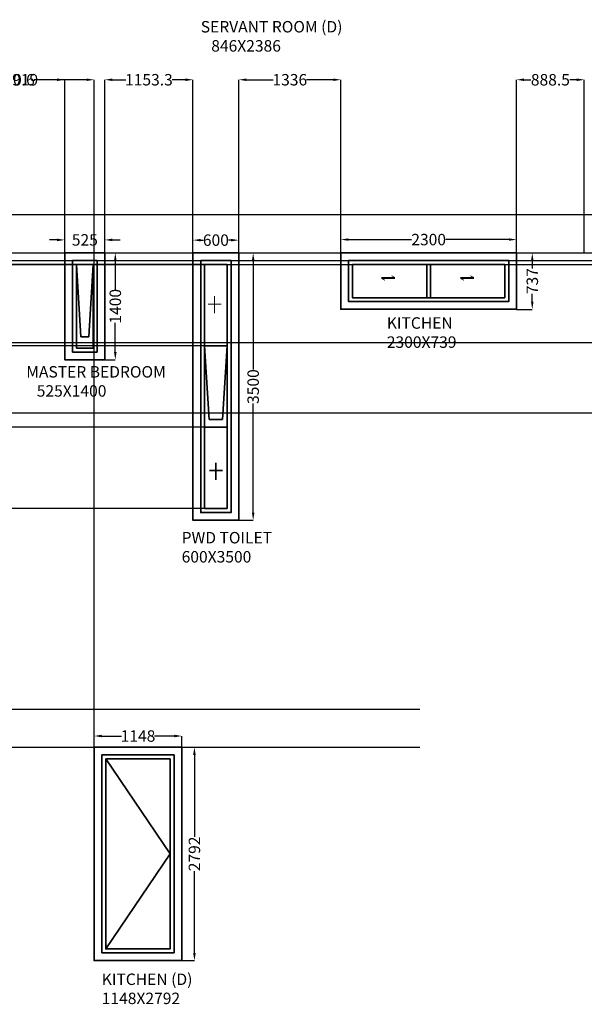
# Model space of a CAD drawing. Units: millimetres. Extents: x 16338 to 57165, y -4429 to 26237.
# Tile 2 of 6: x 24645 to 32038, y -3000 to 9886. Entities that reach past the tile are written whole.
import ezdxf

# ---------------------------------------------------------------- set-up
doc = ezdxf.new("R2010")
doc.units = ezdxf.units.MM
doc.header["$MEASUREMENT"] = 0
for name, color, linetype, lineweight in [('A-ANNO-DIMS', 5, 'Continuous', 18), ('A-ANNO-SYMB', 4, 'Continuous', 18), ('A-ANNO-TEXT', 3, 'Continuous', 18), ('A-ELEV', 8, 'Continuous', 25), ('A-GLAZ', 7, 'Continuous', 35)]:
    doc.layers.add(name, color=color, linetype=linetype, lineweight=lineweight)
doc.styles.get("Standard").update_dxf_attribs({"font": 'arial.ttf'})
doc.dimstyles.get("Standard").update_dxf_attribs({"dimtxt": 150, "dimasz": 100, "dimexe": 0.18, "dimexo": 0.0625, "dimgap": 0.09, "dimtad": 0, "dimdec": 0, "dimzin": 0, "dimdsep": 46, "dimtxsty": 'Standard', "dimcen": 0.09, "dimadec": 0, "dimazin": 0, "dimtfac": 1, "dimtdec": 0, "dimtofl": 0, "dimtmove": 0, "dimatfit": 3, "dimfxl": 1, "dimtolj": 1, "dimtzin": 0, "dimarcsym": 0})

# ---------------------------------------------------------------- blocks, each defined once
blk = doc.blocks.new('*D54')
at = {"layer": 'A-ANNO-DIMS', "color": 0, "lineweight": -2, "transparency": 16777216}
for p, q in [((25135, 7004), (25035, 7004)), ((25235, 6835), (25235, 7004)), ((25760, 6834), (25760, 7004)), ((25860, 7004), (25960, 7004))]:
    blk.add_line(p, q, dxfattribs=at)
at = {"layer": 'A-ANNO-DIMS', "color": 0, "transparency": 16777216}
for points in [[(25135, 7021), (25135, 6987), (25235, 7004)], [(25860, 7021), (25860, 6987), (25760, 7004)]]:
    blk.add_solid(points, dxfattribs=at)
at = {"layer": 'Defpoints', "color": 0, "transparency": 16777216}
for p in [(25760, 7004), (25235, 6835), (25760, 6834)]:
    blk.add_point(p, dxfattribs=at)
at = {"layer": 'A-ANNO-DIMS', "color": 0, "transparency": 16777216, "insert": (25498, 7004), "char_height": 150, "attachment_point": 5}
blk.add_mtext('\\A1;525', dxfattribs=at)
blk = doc.blocks.new('*D55')
at = {"layer": 'A-ANNO-DIMS', "color": 0, "lineweight": -2, "transparency": 16777216}
for p, q in [((25760, 6835), (25897, 6835)), ((25897, 6735), (25897, 6352)), ((25897, 5535), (25897, 5918)), ((25760, 5435), (25897, 5435))]:
    blk.add_line(p, q, dxfattribs=at)
at = {"layer": 'A-ANNO-DIMS', "color": 0, "transparency": 16777216}
for points in [[(25880, 6735), (25914, 6735), (25897, 6835)], [(25880, 5535), (25914, 5535), (25897, 5435)]]:
    blk.add_solid(points, dxfattribs=at)
at = {"layer": 'Defpoints', "color": 0, "transparency": 16777216}
for p in [(25760, 6835), (25760, 5435), (25897, 5435)]:
    blk.add_point(p, dxfattribs=at)
at = {"layer": 'A-ANNO-DIMS', "color": 0, "transparency": 16777216, "insert": (25897, 6135), "char_height": 150, "attachment_point": 5, "rotation": 90}
blk.add_mtext('\\A1;1400', dxfattribs=at)
blk = doc.blocks.new('*D56')
at = {"layer": 'A-ANNO-DIMS', "color": 0, "lineweight": -2, "transparency": 16777216}
for p, q in [((26914, 6835), (26914, 7001)), ((27014, 7001), (27048, 7001)), ((27414, 7001), (27380, 7001)), ((27514, 6835), (27514, 7001))]:
    blk.add_line(p, q, dxfattribs=at)
at = {"layer": 'A-ANNO-DIMS', "color": 0, "transparency": 16777216}
for points in [[(27014, 7017), (27014, 6984), (26914, 7001)], [(27414, 7017), (27414, 6984), (27514, 7001)]]:
    blk.add_solid(points, dxfattribs=at)
at = {"layer": 'Defpoints', "color": 0, "transparency": 16777216}
for p in [(27514, 7001), (26914, 6834), (27514, 6834)]:
    blk.add_point(p, dxfattribs=at)
at = {"layer": 'A-ANNO-DIMS', "color": 0, "transparency": 16777216, "insert": (27214, 7001), "char_height": 150, "attachment_point": 5}
blk.add_mtext('\\A1;600', dxfattribs=at)
blk = doc.blocks.new('*D57')
at = {"layer": 'A-ANNO-DIMS', "color": 0, "lineweight": -2, "transparency": 16777216}
for p, q in [((27514, 6834), (27703, 6834)), ((27702, 6734), (27702, 5308)), ((27702, 3434), (27702, 4861)), ((27514, 3334), (27703, 3334))]:
    blk.add_line(p, q, dxfattribs=at)
at = {"layer": 'A-ANNO-DIMS', "color": 0, "transparency": 16777216}
for points in [[(27686, 6734), (27719, 6734), (27702, 6834)], [(27686, 3434), (27719, 3434), (27702, 3334)]]:
    blk.add_solid(points, dxfattribs=at)
at = {"layer": 'Defpoints', "color": 0, "transparency": 16777216}
for p in [(27514, 6834), (27514, 3334), (27702, 3334)]:
    blk.add_point(p, dxfattribs=at)
at = {"layer": 'A-ANNO-DIMS', "color": 0, "transparency": 16777216, "insert": (27702, 5084), "char_height": 150, "attachment_point": 5, "rotation": 90}
blk.add_mtext('\\A1;3500', dxfattribs=at)
blk = doc.blocks.new('*D58')
at = {"layer": 'A-ANNO-DIMS', "color": 0, "lineweight": -2, "transparency": 16777216}
for p, q in [((28850, 6834), (28850, 7008)), ((28950, 7008), (29775, 7008)), ((31050, 7008), (30225, 7008)), ((31150, 6834), (31150, 7008))]:
    blk.add_line(p, q, dxfattribs=at)
at = {"layer": 'A-ANNO-DIMS', "color": 0, "transparency": 16777216}
for points in [[(28950, 7025), (28950, 6992), (28850, 7008)], [(31050, 7025), (31050, 6992), (31150, 7008)]]:
    blk.add_solid(points, dxfattribs=at)
at = {"layer": 'Defpoints', "color": 0, "transparency": 16777216}
for p in [(31150, 7008), (28850, 6834), (31150, 6834)]:
    blk.add_point(p, dxfattribs=at)
at = {"layer": 'A-ANNO-DIMS', "color": 0, "transparency": 16777216, "insert": (30000, 7008), "char_height": 150, "attachment_point": 5}
blk.add_mtext('\\A1;2300', dxfattribs=at)
blk = doc.blocks.new('*D75')
at = {"layer": 'A-ANNO-DIMS', "color": 0, "lineweight": -2, "transparency": 16777216}
for p, q in [((25620, 364), (25620, 511)), ((25720, 511), (25977, 511)), ((26668, 511), (26411, 511)), ((26768, 364), (26768, 511))]:
    blk.add_line(p, q, dxfattribs=at)
at = {"layer": 'A-ANNO-DIMS', "color": 0, "transparency": 16777216}
for points in [[(25720, 528), (25720, 494), (25620, 511)], [(26668, 528), (26668, 494), (26768, 511)]]:
    blk.add_solid(points, dxfattribs=at)
at = {"layer": 'Defpoints', "color": 0, "transparency": 16777216}
for p in [(26768, 511), (25620, 364), (26768, 364)]:
    blk.add_point(p, dxfattribs=at)
at = {"layer": 'A-ANNO-DIMS', "color": 0, "transparency": 16777216, "insert": (26194, 511), "char_height": 150, "attachment_point": 5}
blk.add_mtext('\\A1;1148', dxfattribs=at)
blk = doc.blocks.new('*D76')
at = {"layer": 'A-ANNO-DIMS', "color": 0, "lineweight": -2, "transparency": 16777216}
for p, q in [((26768, 364), (26933, 364)), ((26933, 264), (26933, -807)), ((26933, -2328), (26933, -1256)), ((26768, -2428), (26933, -2428))]:
    blk.add_line(p, q, dxfattribs=at)
at = {"layer": 'A-ANNO-DIMS', "color": 0, "transparency": 16777216}
for points in [[(26916, 264), (26950, 264), (26933, 364)], [(26916, -2328), (26950, -2328), (26933, -2428)]]:
    blk.add_solid(points, dxfattribs=at)
at = {"layer": 'Defpoints', "color": 0, "transparency": 16777216}
for p in [(26768, 364), (26768, -2428), (26933, -2428)]:
    blk.add_point(p, dxfattribs=at)
at = {"layer": 'A-ANNO-DIMS', "color": 0, "transparency": 16777216, "insert": (26933, -1032), "char_height": 150, "attachment_point": 5, "rotation": 90}
blk.add_mtext('\\A1;2792', dxfattribs=at)
blk = doc.blocks.new('*D78')
at = {"layer": 'A-ANNO-DIMS', "color": 0, "lineweight": -2, "transparency": 16777216}
for p, q in [((31150, 6833), (31357, 6833)), ((31357, 6733), (31357, 6629)), ((31357, 6195), (31357, 6299)), ((31150, 6095), (31357, 6095))]:
    blk.add_line(p, q, dxfattribs=at)
at = {"layer": 'A-ANNO-DIMS', "color": 0, "transparency": 16777216}
for points in [[(31340, 6733), (31373, 6733), (31357, 6833)], [(31340, 6195), (31373, 6195), (31357, 6095)]]:
    blk.add_solid(points, dxfattribs=at)
at = {"layer": 'Defpoints', "color": 0, "transparency": 16777216}
for p in [(31150, 6833), (31150, 6095), (31357, 6095)]:
    blk.add_point(p, dxfattribs=at)
at = {"layer": 'A-ANNO-DIMS', "color": 0, "transparency": 16777216, "insert": (31357, 6464), "char_height": 150, "attachment_point": 5, "rotation": 90}
blk.add_mtext('\\A1;737', dxfattribs=at)
blk = doc.blocks.new('SLIDE-ARROW-S')
for p, q in [((173, 0), (132, 24)), ((0, 0), (173, 0))]:
    blk.add_line(p, q)
blk = doc.blocks.new('*D109')
at = {"layer": 'A-ANNO-DIMS', "color": 0, "lineweight": -2, "transparency": 16777216}
for p, q in [((23825, 6835), (23825, 9100)), ((23925, 9100), (24226, 9100)), ((25135, 9100), (24834, 9100)), ((25235, 6835), (25235, 9100))]:
    blk.add_line(p, q, dxfattribs=at)
at = {"layer": 'A-ANNO-DIMS', "color": 0, "transparency": 16777216}
for points in [[(23925, 9117), (23925, 9083), (23825, 9100)], [(25135, 9117), (25135, 9083), (25235, 9100)]]:
    blk.add_solid(points, dxfattribs=at)
at = {"layer": 'Defpoints', "color": 0, "transparency": 16777216}
for p in [(25235, 9100), (23825, 6835), (25235, 6835)]:
    blk.add_point(p, dxfattribs=at)
at = {"layer": 'A-ANNO-DIMS', "color": 0, "transparency": 16777216, "insert": (24530, 9100), "char_height": 150, "attachment_point": 5}
blk.add_mtext('\\A1;1410.6', dxfattribs=at)
blk = doc.blocks.new('*D110')
at = {"layer": 'A-ANNO-DIMS', "color": 0, "lineweight": -2, "transparency": 16777216}
for p, q in [((25760, 6835), (25760, 9100)), ((25860, 9100), (26033, 9100)), ((26814, 9100), (26641, 9100)), ((26914, 6835), (26914, 9100))]:
    blk.add_line(p, q, dxfattribs=at)
at = {"layer": 'A-ANNO-DIMS', "color": 0, "transparency": 16777216}
for points in [[(25860, 9117), (25860, 9083), (25760, 9100)], [(26814, 9117), (26814, 9083), (26914, 9100)]]:
    blk.add_solid(points, dxfattribs=at)
at = {"layer": 'Defpoints', "color": 0, "transparency": 16777216}
for p in [(26914, 9100), (25760, 6835), (26914, 6834)]:
    blk.add_point(p, dxfattribs=at)
at = {"layer": 'A-ANNO-DIMS', "color": 0, "transparency": 16777216, "insert": (26337, 9100), "char_height": 150, "attachment_point": 5}
blk.add_mtext('\\A1;1153.3', dxfattribs=at)
blk = doc.blocks.new('*D111')
at = {"layer": 'A-ANNO-DIMS', "color": 0, "lineweight": -2, "transparency": 16777216}
for p, q in [((27514, 6835), (27514, 9100)), ((27614, 9100), (27965, 9100)), ((28750, 9100), (28399, 9100)), ((28850, 6834), (28850, 9100))]:
    blk.add_line(p, q, dxfattribs=at)
at = {"layer": 'A-ANNO-DIMS', "color": 0, "transparency": 16777216}
for points in [[(27614, 9117), (27614, 9083), (27514, 9100)], [(28750, 9117), (28750, 9083), (28850, 9100)]]:
    blk.add_solid(points, dxfattribs=at)
at = {"layer": 'Defpoints', "color": 0, "transparency": 16777216}
for p in [(28850, 9100), (27514, 6834), (28850, 6834)]:
    blk.add_point(p, dxfattribs=at)
at = {"layer": 'A-ANNO-DIMS', "color": 0, "transparency": 16777216, "insert": (28182, 9100), "char_height": 150, "attachment_point": 5}
blk.add_mtext('\\A1;1336', dxfattribs=at)
blk = doc.blocks.new('*D112')
at = {"layer": 'A-ANNO-DIMS', "color": 0, "lineweight": -2, "transparency": 16777216}
for p, q in [((31150, 6834), (31150, 9100)), ((31250, 9100), (31340, 9100)), ((31938, 9100), (31848, 9100)), ((32038, 6835), (32038, 9100))]:
    blk.add_line(p, q, dxfattribs=at)
at = {"layer": 'A-ANNO-DIMS', "color": 0, "transparency": 16777216}
for points in [[(31250, 9117), (31250, 9083), (31150, 9100)], [(31938, 9117), (31938, 9083), (32038, 9100)]]:
    blk.add_solid(points, dxfattribs=at)
at = {"layer": 'Defpoints', "color": 0, "transparency": 16777216}
for p in [(32038, 9100), (31150, 6834), (32038, 6835)]:
    blk.add_point(p, dxfattribs=at)
at = {"layer": 'A-ANNO-DIMS', "color": 0, "transparency": 16777216, "insert": (31594, 9100), "char_height": 150, "attachment_point": 5}
blk.add_mtext('\\A1;888.5', dxfattribs=at)
blk = doc.blocks.new('*D119')
at = {"layer": 'A-ANNO-DIMS', "color": 0, "lineweight": -2, "transparency": 16777216}
for p, q in [((23701, 364), (23701, 9100)), ((23801, 9100), (24443, 9100)), ((25520, 9100), (24877, 9100)), ((25620, 364), (25620, 9100))]:
    blk.add_line(p, q, dxfattribs=at)
at = {"layer": 'A-ANNO-DIMS', "color": 0, "transparency": 16777216}
for points in [[(23801, 9117), (23801, 9083), (23701, 9100)], [(25520, 9117), (25520, 9083), (25620, 9100)]]:
    blk.add_solid(points, dxfattribs=at)
at = {"layer": 'Defpoints', "color": 0, "transparency": 16777216}
for p in [(25620, 9100), (23701, 364), (25620, 364)]:
    blk.add_point(p, dxfattribs=at)
at = {"layer": 'A-ANNO-DIMS', "color": 0, "transparency": 16777216, "insert": (24660, 9100), "char_height": 150, "attachment_point": 5}
blk.add_mtext('\\A1;1919', dxfattribs=at)
blk = doc.blocks.new('*D121')
at = {"layer": 'A-ANNO-DIMS', "color": 0, "lineweight": -2, "transparency": 16777216}
for p, q in [((27066, 6682), (16437, 6682)), ((16437, 6582), (16437, 6367)), ((16437, 5717), (16437, 5932)), ((27066, 5617), (16437, 5617))]:
    blk.add_line(p, q, dxfattribs=at)
at = {"layer": 'A-ANNO-DIMS', "color": 0, "transparency": 16777216}
for points in [[(16420, 6582), (16454, 6582), (16437, 6682)], [(16420, 5717), (16454, 5717), (16437, 5617)]]:
    blk.add_solid(points, dxfattribs=at)
at = {"layer": 'Defpoints', "color": 0, "transparency": 16777216}
for p in [(27066, 6682), (16437, 5617), (27066, 5617)]:
    blk.add_point(p, dxfattribs=at)
at = {"layer": 'A-ANNO-DIMS', "color": 0, "transparency": 16777216, "insert": (16437, 6150), "char_height": 150, "attachment_point": 5, "rotation": 90}
blk.add_mtext('\\A1;1065', dxfattribs=at)
blk = doc.blocks.new('*D122')
at = {"layer": 'A-ANNO-DIMS', "color": 0, "lineweight": -2, "transparency": 16777216}
for p, q in [((27066, 5617), (16437, 5617)), ((16437, 5517), (16437, 5302)), ((16437, 4652), (16437, 4867)), ((27066, 4552), (16437, 4552))]:
    blk.add_line(p, q, dxfattribs=at)
at = {"layer": 'A-ANNO-DIMS', "color": 0, "transparency": 16777216}
for points in [[(16420, 5517), (16454, 5517), (16437, 5617)], [(16420, 4652), (16454, 4652), (16437, 4552)]]:
    blk.add_solid(points, dxfattribs=at)
at = {"layer": 'Defpoints', "color": 0, "transparency": 16777216}
for p in [(27066, 5617), (16437, 4552), (27066, 4552)]:
    blk.add_point(p, dxfattribs=at)
at = {"layer": 'A-ANNO-DIMS', "color": 0, "transparency": 16777216, "insert": (16437, 5084), "char_height": 150, "attachment_point": 5, "rotation": 90}
blk.add_mtext('\\A1;1065', dxfattribs=at)
blk = doc.blocks.new('*D123')
at = {"layer": 'A-ANNO-DIMS', "color": 0, "lineweight": -2, "transparency": 16777216}
for p, q in [((27066, 4552), (16437, 4552)), ((16437, 4452), (16437, 4237)), ((16437, 3587), (16437, 3802)), ((27066, 3487), (16437, 3487))]:
    blk.add_line(p, q, dxfattribs=at)
at = {"layer": 'A-ANNO-DIMS', "color": 0, "transparency": 16777216}
for points in [[(16420, 4452), (16454, 4452), (16437, 4552)], [(16420, 3587), (16454, 3587), (16437, 3487)]]:
    blk.add_solid(points, dxfattribs=at)
at = {"layer": 'Defpoints', "color": 0, "transparency": 16777216}
for p in [(27066, 4552), (16437, 3487), (27066, 3487)]:
    blk.add_point(p, dxfattribs=at)
at = {"layer": 'A-ANNO-DIMS', "color": 0, "transparency": 16777216, "insert": (16437, 4019), "char_height": 150, "attachment_point": 5, "rotation": 90}
blk.add_mtext('\\A1;1065', dxfattribs=at)
blk = doc.blocks.new('*D126')
at = {"layer": 'A-ANNO-DIMS', "color": 0, "lineweight": -2, "transparency": 16777216}
for p, q in [((52648, 6935), (52648, 7035)), ((23825, 6835), (52648, 6835)), ((23725, 6735), (52648, 6735)), ((52648, 6635), (52648, 6535))]:
    blk.add_line(p, q, dxfattribs=at)
at = {"layer": 'A-ANNO-DIMS', "color": 0, "transparency": 16777216}
for points in [[(52631, 6935), (52665, 6935), (52648, 6835)], [(52631, 6635), (52665, 6635), (52648, 6735)]]:
    blk.add_solid(points, dxfattribs=at)
at = {"layer": 'Defpoints', "color": 0, "transparency": 16777216}
for p in [(23825, 6835), (23725, 6735), (52648, 6735)]:
    blk.add_point(p, dxfattribs=at)
at = {"layer": 'A-ANNO-DIMS', "color": 0, "transparency": 16777216, "insert": (52648, 6377), "char_height": 150, "attachment_point": 5, "rotation": 90}
blk.add_mtext('\\A1;100', dxfattribs=at)
blk = doc.blocks.new('*D127')
at = {"layer": 'A-ANNO-DIMS', "color": 0, "lineweight": -2, "transparency": 16777216}
for p, q in [((52648, 6835), (52648, 6935)), ((23725, 6735), (52648, 6735)), ((23674, 6684), (52648, 6684)), ((52648, 6584), (52648, 6484))]:
    blk.add_line(p, q, dxfattribs=at)
at = {"layer": 'A-ANNO-DIMS', "color": 0, "transparency": 16777216}
for points in [[(52631, 6835), (52665, 6835), (52648, 6735)], [(52631, 6584), (52665, 6584), (52648, 6684)]]:
    blk.add_solid(points, dxfattribs=at)
at = {"layer": 'Defpoints', "color": 0, "transparency": 16777216}
for p in [(23725, 6735), (23674, 6684), (52648, 6684)]:
    blk.add_point(p, dxfattribs=at)
at = {"layer": 'A-ANNO-DIMS', "color": 0, "transparency": 16777216, "insert": (52648, 6289), "char_height": 150, "attachment_point": 5, "rotation": 90}
blk.add_mtext('\\A1;50.8', dxfattribs=at)
blk = doc.blocks.new('*D132')
at = {"layer": 'A-ANNO-DIMS', "color": 0, "lineweight": -2, "transparency": 16777216}
for p, q in [((23674, 5663), (52648, 5663)), ((52648, 5563), (52648, 5441)), ((52648, 4842), (52648, 4964)), ((23616, 4742), (52648, 4742))]:
    blk.add_line(p, q, dxfattribs=at)
at = {"layer": 'A-ANNO-DIMS', "color": 0, "transparency": 16777216}
for points in [[(52631, 5563), (52665, 5563), (52648, 5663)], [(52631, 4842), (52665, 4842), (52648, 4742)]]:
    blk.add_solid(points, dxfattribs=at)
at = {"layer": 'Defpoints', "color": 0, "transparency": 16777216}
for p in [(23674, 5663), (52648, 5663), (23616, 4742)]:
    blk.add_point(p, dxfattribs=at)
at = {"layer": 'A-ANNO-DIMS', "color": 0, "transparency": 16777216, "insert": (52648, 5203), "char_height": 150, "attachment_point": 5, "rotation": 90}
blk.add_mtext('\\A1;921.1', dxfattribs=at)

msp = doc.modelspace()

# ---------------------------------------------------------------- linework, layer by layer
at = {"layer": 'A-ANNO-DIMS'}
for p in [(27361.18, 5617), (27361.18, 4551.93)]:
    msp.add_point(p, dxfattribs=at)
at = {"layer": 'A-ANNO-SYMB'}
for p, q in [((27197.57, 6043.31), (27197.57, 6265.76)), ((27112.65, 6162.56), (27282.5, 6162.56))]:
    msp.add_line(p, q, dxfattribs=at)
at = {"layer": 'A-ELEV'}
for p, q in [((18209.23, 7335.1), (50757.08, 7335.1)), ((18201.83, 6834.85), (50882.91, 6829.39)), ((18334.8, 864.14), (29883.27, 864.14)), ((18334.8, 364.14), (29883.27, 364.14))]:
    msp.add_line(p, q, dxfattribs=at)
at = {"layer": 'A-GLAZ'}
for p, q in [((25387.63, 6682.7), (25607.83, 6682.7)), ((25387.63, 5587.5), (25387.63, 6682.7)), ((25387.63, 6682.7), (25446.54, 5737.5)), ((25607.83, 6682.7), (25548.93, 5737.5)), ((25607.83, 6682.7), (25607.83, 5587.5)), ((27065.98, 6682.06), (27361.18, 6682.06)), ((27065.98, 3486.86), (27065.98, 6682.06)), ((27361.18, 6682.06), (27361.18, 3486.86)), ((29974.22, 6682), (29974.22, 6247.8)), ((30025.02, 6682), (30025.02, 6247.8)), ((25548.93, 5737.5), (25446.54, 5737.5)), ((25607.83, 5587.5), (25387.63, 5587.5)), ((27361.18, 5617), (27065.98, 5617)), ((27065.98, 5617), (27127.29, 4651.93)), ((27361.18, 5617), (27299.87, 4651.93)), ((27299.87, 4651.93), (27127.29, 4651.93)), ((27361.18, 4551.93), (27065.98, 4551.93)), ((27213.63, 3865.04), (27213.63, 4087.49)), ((27128.7, 3984.29), (27298.55, 3984.29)), ((27361.18, 3486.86), (27065.98, 3486.86)), ((25772.15, 211.74), (26615.35, -1031.86)), ((26615.35, -1031.86), (25772.15, -2275.46))]:
    msp.add_line(p, q, dxfattribs=at)
for points in [[(25235.23, 6835.1), (25760.23, 6835.1), (25760.23, 5435.1), (25235.23, 5435.1)], [(26913.58, 6834.46), (27513.58, 6834.46), (27513.58, 3334.46), (26913.58, 3334.46)], [(28849.62, 6834.4), (31149.62, 6834.4), (31149.62, 6095.4), (28849.62, 6095.4)], [(25336.83, 6733.5), (25658.63, 6733.5), (25658.63, 5536.7), (25336.83, 5536.7)], [(27015.18, 6732.86), (27411.98, 6732.86), (27411.98, 3436.06), (27015.18, 3436.06)], [(28951.22, 6732.8), (31048.02, 6732.8), (31048.02, 6197), (28951.22, 6197)], [(29002.02, 6682), (30997.22, 6682), (30997.22, 6247.8), (29002.02, 6247.8)], [(25619.75, 364.14), (26767.75, 364.14), (26767.75, -2427.86), (25619.75, -2427.86)], [(25721.35, 262.54), (26666.15, 262.54), (26666.15, -2326.26), (25721.35, -2326.26)], [(25772.15, 211.74), (26615.35, 211.74), (26615.35, -2275.46), (25772.15, -2275.46)]]:
    msp.add_lwpolyline(points, close=True, dxfattribs=at)

# ---------------------------------------------------------------- block references
at = {"layer": 'A-ANNO-SYMB'}
for p in [(29384.25, 6510), (30417.18, 6510)]:
    msp.add_blockref('SLIDE-ARROW-S', p, dxfattribs=at)
at = {"layer": 'A-ANNO-SYMB', "rotation": 180}
for p in [(29557.56, 6500.59), (30590.49, 6500.59)]:
    msp.add_blockref('SLIDE-ARROW-S', p, dxfattribs=at)

# ---------------------------------------------------------------- texts
at = {"layer": 'A-ANNO-TEXT', "char_height": 150, "attachment_point": 1}
for s, insert in [('SERVANT ROOM (D)\\P   846X2386', (27015.82, 9868.61)), ('KITCHEN\\P2300X739', (29452.18, 5991.32)), ('MASTER BEDROOM\\P   525X1400', (24731.03, 5352.41)), ('PWD TOILET\\P600X3500', (26765.78, 3181.71)), ('KITCHEN (D)\\P1148X2792', (25719.62, -2597.76))]:
    msp.add_mtext_dynamic_manual_height_columns(s, width=7094.9176, gutter_width=1, heights=[0], dxfattribs=dict(at, insert=insert))

# ---------------------------------------------------------------- dimensions: what is measured, and where the dimension line sits
at = {"layer": 'A-ANNO-DIMS'}
for base, p1, p2, override, picture, middle in [((25619.75, 9100.1), (23700.67, 364.14), (25619.75, 364.14), {"dimdec": 0, "dimlfac": 1, "dimrnd": 0, "dimzin": 0, "dimdsep": 46, "dimlunit": 2}, '*D119', (24660.21, 9100.1)), ((25235.23, 9100.1), (23824.59, 6835.1), (25235.23, 6835.1), {"dimdec": 1, "dimlfac": 1, "dimrnd": 0, "dimzin": 0, "dimdsep": 46, "dimlunit": 2}, '*D109', (24529.91, 9100.1)), ((26913.5755, 9100.1048), (25760.2334, 6835.1048), (26913.5755, 6834.4635), {"dimdec": 1, "dimlfac": 1, "dimrnd": 0, "dimzin": 0, "dimdsep": 46, "dimlunit": 2}, '*D110', (26336.9044, 9100.1048)), ((28849.62, 9100.1), (27513.58, 6834.46), (28849.62, 6834.4), {"dimdec": 0, "dimlfac": 1, "dimrnd": 0, "dimzin": 0, "dimdsep": 46, "dimlunit": 2}, '*D111', (28181.6, 9100.1)), ((32038.13, 9100.1), (31149.62, 6834.4), (32038.13, 6835.1), {"dimdec": 1, "dimlfac": 1, "dimrnd": 0, "dimzin": 0, "dimdsep": 46, "dimlunit": 2}, '*D112', (31593.88, 9100.1)), ((25760.23, 7004.15), (25235.23, 6835.1), (25760.23, 6833.59), {"dimclrd": 0, "dimclre": 0, "dimclrt": 0}, '*D54', (25497.73, 7004.15)), ((27513.58, 7000.63), (26913.58, 6834.46), (27513.58, 6834.46), {"dimclrd": 0, "dimclre": 0, "dimclrt": 0}, '*D56', (27213.58, 7000.63)), ((31149.62, 7008.21), (28849.62, 6834.4), (31149.62, 6834.4), {"dimclrd": 0, "dimclre": 0, "dimclrt": 0}, '*D58', (29999.62, 7008.21)), ((26767.75, 511.1), (25619.75, 364.14), (26767.75, 364.14), {"dimclrd": 0, "dimclre": 0, "dimclrt": 0}, '*D75', (26193.75, 511.1))]:
    dim = msp.add_linear_dim(base=base, p1=p1, p2=p2, dimstyle='Standard', override=override, dxfattribs=at)
    dim.commit()
    dim.dimension.update_dxf_attribs({"geometry": picture, "text_midpoint": middle})
for base, p1, p2, override, picture, middle in [((52647.91, 6735.1), (23824.59, 6835.1), (23724.59, 6735.1), {"dimdec": 0, "dimlfac": 1, "dimrnd": 0, "dimzin": 0, "dimdsep": 46, "dimlunit": 2}, '*D126', (52647.91, 6376.62)), ((52647.91, 6684.3), (23724.59, 6735.1), (23673.79, 6684.3), {"dimdec": 1, "dimlfac": 1, "dimrnd": 0, "dimzin": 0, "dimdsep": 46, "dimlunit": 2}, '*D127', (52647.91, 6289.25)), ((25896.88, 5435.1), (25760.23, 6835.1), (25760.23, 5435.1), {"dimclrd": 0, "dimclre": 0, "dimclrt": 0}, '*D55', (25896.88, 6135.1)), ((27702.39, 3334.46), (27513.58, 6834.46), (27513.58, 3334.46), {"dimclrd": 0, "dimclre": 0, "dimclrt": 0}, '*D57', (27702.39, 5084.46)), ((31356.56, 6095.4), (31149.62, 6832.69), (31149.62, 6095.4), {"dimclrd": 0, "dimclre": 0, "dimclrt": 0}, '*D78', (31356.56, 6464.04)), ((16436.83, 5617), (27065.98, 6682.06), (27065.98, 5617), {"dimdec": 0, "dimlfac": 1, "dimrnd": 0, "dimzin": 0, "dimdsep": 46, "dimlunit": 2}, '*D121', (16436.83, 6149.53)), ((16436.83, 4551.93), (27065.98, 5617), (27065.98, 4551.93), {"dimdec": 0, "dimlfac": 1, "dimrnd": 0, "dimzin": 0, "dimdsep": 46, "dimlunit": 2}, '*D122', (16436.83, 5084.46)), ((52647.91, 5663.17), (23615.55, 4742.04), (23673.79, 5663.17), {"dimdec": 1, "dimlfac": 1, "dimrnd": 0, "dimzin": 0, "dimdsep": 46, "dimlunit": 2}, '*D132', (52647.91, 5202.6)), ((16436.83, 3486.86), (27065.98, 4551.93), (27065.98, 3486.86), {"dimdec": 0, "dimlfac": 1, "dimrnd": 0, "dimzin": 0, "dimdsep": 46, "dimlunit": 2}, '*D123', (16436.83, 4019.4)), ((26933.05, -2427.86), (26767.75, 364.14), (26767.75, -2427.86), {"dimclrd": 0, "dimclre": 0, "dimclrt": 0}, '*D76', (26933.05, -1031.86))]:
    dim = msp.add_linear_dim(base=base, p1=p1, p2=p2, angle=90, dimstyle='Standard', override=override, dxfattribs=at)
    dim.commit()
    dim.dimension.update_dxf_attribs({"geometry": picture, "text_midpoint": middle})

doc.saveas('drawing.dxf')
